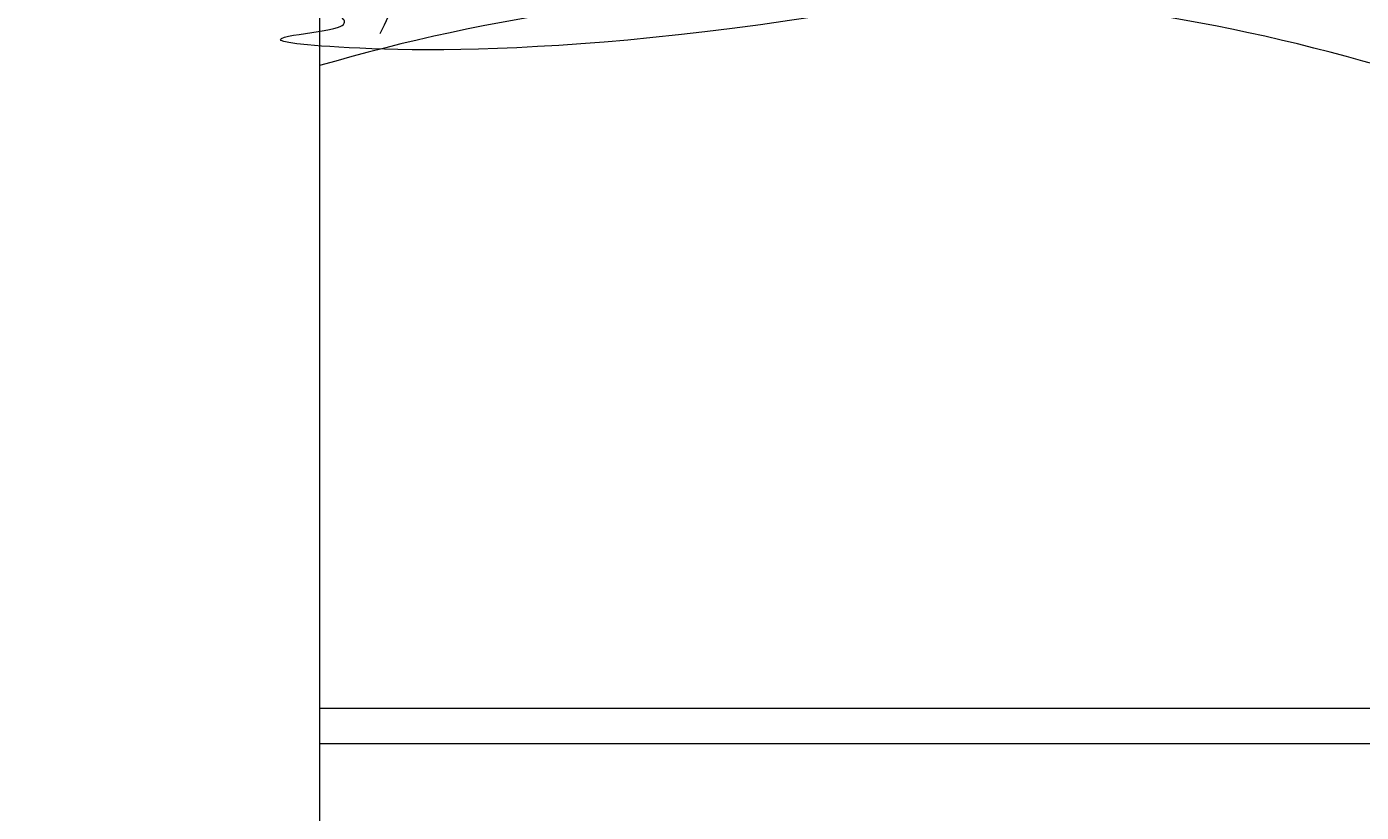
# Model space of a CAD drawing. Units: inches. Extents: x -61 to 1599, y -1316 to 257.
# Tile 35 of 204: x 91 to 134, y -763 to -738. Entities that reach past the tile are written whole.
import ezdxf

# ---------------------------------------------------------------- set-up
doc = ezdxf.new("R2010")
doc.units = ezdxf.units.IN
doc.header["$MEASUREMENT"] = 0
doc.layers.add('A-ANNO-DIMS', color=2, linetype='Continuous', lineweight=18)
doc.layers.add('FURNITURE', color=83, linetype='Continuous', lineweight=18)
doc.styles.get("Standard").update_dxf_attribs({"font": 'arial.ttf'})
doc.dimstyles.get("Standard").update_dxf_attribs({"dimtxt": 0.18, "dimasz": 0.18, "dimexe": 0.18, "dimexo": 0.0625, "dimgap": 0.09, "dimtad": 0, "dimtih": 1, "dimtoh": 1, "dimdec": 0, "dimzin": 0, "dimdsep": 46, "dimlunit": 3, "dimtxsty": 'Standard', "dimcen": 0.09, "dimadec": 0, "dimazin": 0, "dimtfac": 1, "dimtdec": 0, "dimtofl": 0, "dimtmove": 0, "dimatfit": 3, "dimfxl": 1, "dimtolj": 1, "dimtzin": 0, "dimarcsym": 0})

# ---------------------------------------------------------------- blocks, each defined once
blk = doc.blocks.new('BED-DOUBLE')
for p, q in [((1.272, 20.467), (70.263, 20.467)), ((1.272, 19.317), (70.263, 19.317))]:
    blk.add_line(p, q)
blk.add_lwpolyline([(1.272, 88.537), (1.272, 3.449, 0.414214), (4.722, 0), (66.813, 0, 0.414214), (70.263, 3.449), (70.263, 88.537, 0.414214), (66.813, 91.987), (4.722, 91.987, 0.414214)], format="xyb", close=True)
blk.add_lwpolyline([(70.263, 41.387, -0.22309), (35.767, 41.387, 0.142156), (1.272, 41.387)], format="xyb")
blk.add_rational_spline([(70.263, 57.9), (59.862, 50.943), (48.595, 45.5), (36.681, 41.677), (36.463, 41.771), (36.247, 41.868), (36.032, 41.966), (24.597, 45.284), (12.692, 45.258), (1.272, 41.889), (2.723, 44.9), (5.745, 51.172), (0.137, 60.702), (6.828, 69.972), (0.109, 77.787), (4.354, 84.383), (5.398, 86.876)], [1, 0.993520320424, 0.993520320424, 1, 0.99997444972, 0.99997444972, 1, 0.973174868659, 0.973174868659, 1, 1, 1, 1, 1, 1, 1, 1], degree=3, knots=[0, 0, 0, 0, 0.279074, 0.279074, 0.279074, 0.296584, 0.296584, 0.296584, 0.865868, 0.865868, 0.865868, 9.142578, 18.107734, 25.769226, 34.110801, 40.441511, 40.441511, 40.441511, 40.441511])
blk.add_open_spline([(3.252, 42.437), (4.702, 45.448), (7.724, 51.72), (2.116, 61.25), (8.808, 70.52), (2.434, 77.934), (5.722, 83.908), (6.746, 86.037)], degree=3, knots=[0, 0, 0, 0, 8.27671, 17.241866, 24.903358, 33.244933, 38.427294, 38.427294, 38.427294, 38.427294])
blk = doc.blocks.new('*D687')
at = {"layer": 'A-ANNO-DIMS', "color": 0, "lineweight": -2, "transparency": 16777216}
for p, q in [((289.418, 181.677), (-61.077, 181.677)), ((-60.897, 181.497), (-60.897, -528.952)), ((-60.897, -1239.765), (-60.897, -529.316)), ((319.64, -1239.945), (-61.077, -1239.945))]:
    blk.add_line(p, q, dxfattribs=at)
at = {"layer": 'A-ANNO-DIMS', "color": 0, "transparency": 16777216}
for points in [[(-60.927, 181.497), (-60.867, 181.497), (-60.897, 181.677)], [(-60.927, -1239.765), (-60.867, -1239.765), (-60.897, -1239.945)]]:
    blk.add_solid(points, dxfattribs=at)
at = {"layer": 'DEFPOINTS', "color": 0, "transparency": 16777216}
for p in [(289.481, 181.677), (-60.897, -1239.945), (319.703, -1239.945)]:
    blk.add_point(p, dxfattribs=at)
at = {"layer": 'A-ANNO-DIMS', "color": 0, "transparency": 16777216, "insert": (-60.897, -529.134), "char_height": 0.18, "attachment_point": 5}
blk.add_mtext('\\A1;1421.6', dxfattribs=at)

msp = doc.modelspace()

# ---------------------------------------------------------------- block references
at = {"layer": 'FURNITURE'}
msp.add_blockref('BED-DOUBLE', (98.977, -780.4187), dxfattribs=at)

# ---------------------------------------------------------------- dimensions: what is measured, and where the dimension line sits
at = {"layer": 'A-ANNO-DIMS'}
dim = msp.add_linear_dim(base=(-60.8972, -1239.9446), p1=(289.4807, 181.6771), p2=(319.7028, -1239.9446), angle=90, dimstyle='Standard', override={"dimdec": 1, "dimlfac": 1, "dimrnd": 0, "dimzin": 0, "dimdsep": 46, "dimlunit": 2}, dxfattribs=at)
dim.commit()
dim.dimension.update_dxf_attribs({"geometry": '*D687', "text_midpoint": (-60.8972, -529.1337)})

doc.saveas('drawing.dxf')
